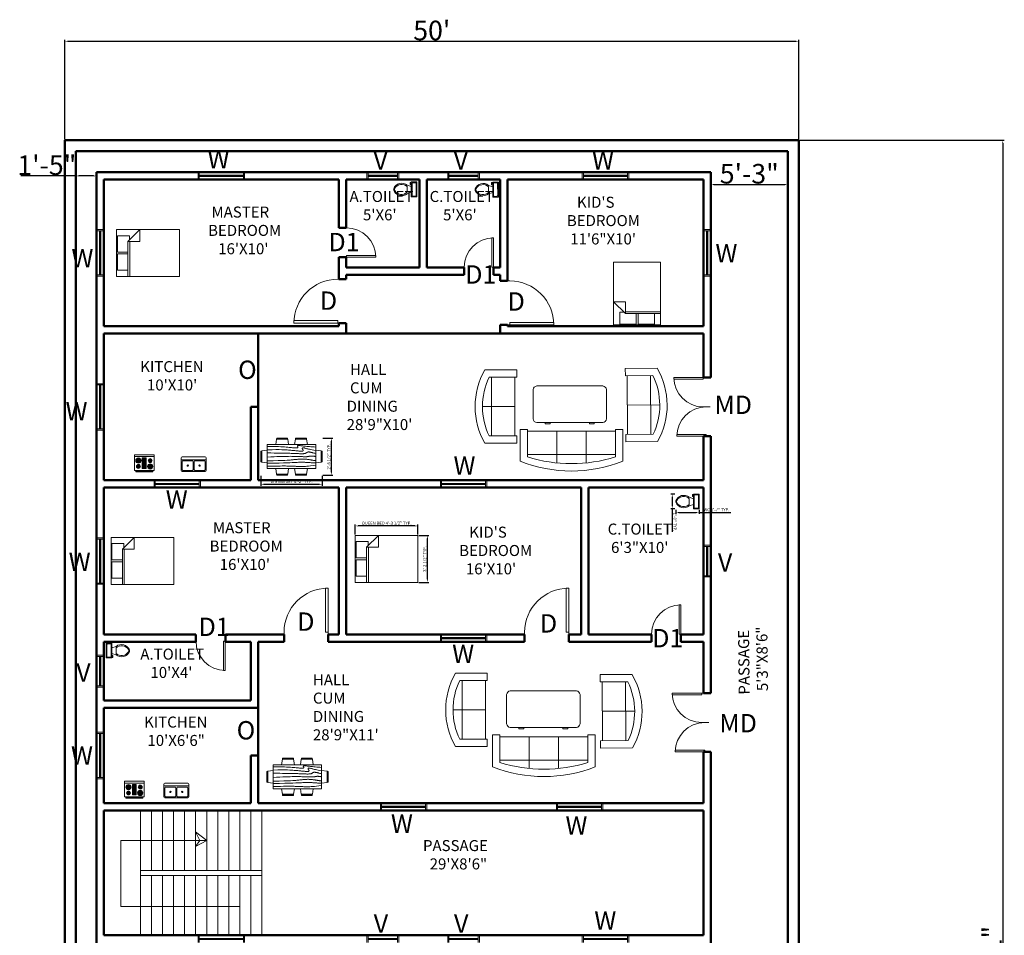
# Model space of a CAD drawing. Units: inches. Extents: x -7040 to -4088, y 6092 to 7645.
# Tile 9 of 11: x -5837 to -5032, y 6864 to 7612. Entities that reach past the tile are written whole.
import ezdxf

# ---------------------------------------------------------------- set-up
doc = ezdxf.new("R2010")
doc.units = ezdxf.units.IN
for name, color, linetype, lineweight in [('A-ANNO-DIMS', 2, 'Continuous', 18), ('A-ANNO-TEXT', 7, 'Continuous', 25), ('A-AREA-IDEN', 3, 'Continuous', 25), ('A-DOOR', 3, 'Continuous', 18), ('A-FLOR-FIXT', 9, 'Continuous', 13), ('A-FLOR-STRS', 2, 'Continuous', 18), ('A-FURN', 8, 'Continuous', 13), ('A-GLAZ', 4, 'Continuous', 18), ('A-WALL', 7, 'Continuous', 50)]:
    doc.layers.add(name, color=color, linetype=linetype, lineweight=lineweight)
doc.styles.get("Standard").update_dxf_attribs({"font": 'arial.ttf'})
doc.dimstyles.new('ISO-25', dxfattribs={"dimtxt": 2.5, "dimasz": 2.5, "dimexe": 1.25, "dimexo": 0.625, "dimtad": 1, "dimdec": 0, "dimlunit": 3, "dimtxsty": 'Standard', "dimcen": 2.5, "dimadec": 0, "dimazin": 0, "dimtfac": 1, "dimtdec": 0, "dimtmove": 0, "dimatfit": 3, "dimfxl": 1, "dimarcsym": 0})

# ---------------------------------------------------------------- blocks, each defined once
blk = doc.blocks.new('*U8')
for p, q in [((0, 0), (0, -100)), ((750, 0), (750, -100))]:
    blk.add_line(p, q)
blk.add_lwpolyline([(0, 0), (0, 750), (43.75, 750), (43.75, 0)], close=True)
blk.add_arc((0, 0), 750, 0, 90)
blk = doc.blocks.new('Bed - Queen')
for p, q in [((0, -80.00003), (0, 0)), ((0, 0), (59.99999, 0)), ((59.99999, 0), (59.99999, -80.00003)), ((7.99999, -1.2), (28.79998, -1.2)), ((7.99999, -14.4), (7.99999, -1.2)), ((28.79998, -1.2), (28.79998, -14.4)), ((31.19999, -1.2), (51.99999, -1.2)), ((31.19999, -14.4), (31.19999, -1.2)), ((51.99999, -1.2), (51.99999, -16.4)), ((0, -14.4), (44.8, -14.4)), ((44.8, -16.8), (0, -16.8)), ((59.99999, -29.6), (44.8, -14.4)), ((44.8, -14.4), (44.8, -29.6)), ((51.99999, -16.4), (46.79936, -16.4)), ((44.8, -29.6), (59.99999, -29.6)), ((59.99999, -80.00003), (0, -80.00003))]:
    blk.add_line(p, q)
blk = doc.blocks.new('Range-Oven - 30 in top')
for p, q in [((0, -3), (30, -3)), ((12, -6), (18, -6)), ((13, -20), (13, -6)), ((14, -6), (14, -20)), ((15, -20), (15, -6)), ((16, -6), (16, -20)), ((17, -20), (17, -6)), ((6, -24), (6, -25)), ((8, -25), (8, -24)), ((18, -20), (12, -20)), ((22, -25), (22, -24)), ((24, -24), (24, -25))]:
    blk.add_line(p, q)
for points in [[(0, -24), (0, 0), (30, 0), (30, -24)], [(12, -21), (12, -5), (18, -5), (18, -21)], [(2, -26), (2, -25), (28, -25), (28, -26)]]:
    blk.add_lwpolyline(points, close=True)
for centre, radius in [((6, -9), 4), ((6, -9), 3), ((6, -18), 3), ((6, -9), 2), ((6, -9), 1), ((24, -18), 4), ((24, -9), 3), ((24, -18), 3), ((24, -9), 2), ((24, -9), 1), ((6, -18), 2), ((6, -18), 1), ((24, -18), 2), ((24, -18), 1)]:
    blk.add_circle(centre, radius)
blk = doc.blocks.new('Sink-double - 36 in top')
for p, q in [((-18, -4), (18, -4)), ((-0.75, -18.5), (-0.75, -6.5)), ((0.75, -6.5), (0.75, -18.5))]:
    blk.add_line(p, q)
for points in [[(-16.5, 0), (16.5, 0)], [(-18, -19.5), (-18, -1.5)], [(-16.5, -18.5), (-16.5, -6.5)], [(-15.5, -5.5), (-1.75, -5.5)], [(1.75, -5.5), (15.5, -5.5)], [(16.5, -6.5), (16.5, -18.5)], [(18, -1.5), (18, -19.5)], [(16.5, -21), (-16.5, -21)], [(-1.75, -19.5), (-15.5, -19.5)], [(15.5, -19.5), (1.75, -19.5)]]:
    blk.add_lwpolyline(points)
for centre, radius in [((-8.5, -12.5), 1), ((-8.5, -12.5), 0.5), ((8.5, -12.5), 1), ((8.5, -12.5), 0.5)]:
    blk.add_circle(centre, radius)
for centre, radius, start, end in [((-16.5, -1.5), 1.5, 90, 180), ((16.5, -1.5), 1.5, 0, 90), ((-15.5, -6.5), 1, 90, 180), ((-1.75, -6.5), 1, 0, 90), ((1.75, -6.5), 1, 90, 180), ((15.5, -6.5), 1, 0, 90), ((-16.5, -19.5), 1.5, 180, 270), ((-15.5, -18.5), 1, 180, 270), ((-1.75, -18.5), 1, 270, 0), ((1.75, -18.5), 1, 180, 270), ((15.5, -18.5), 1, 270, 0), ((16.5, -19.5), 1.5, 270, 0)]:
    blk.add_arc(centre, radius, start, end)
blk = doc.blocks.new('Toilet - top')
for p, q in [((-10, -8.5), (-8, -8.5)), ((-10, -9.5), (-10, -8.5)), ((-7, -9.5), (-10, -9.5)), ((-8, -8.5), (-8, -8)), ((-7, -8), (-7, -9.5)), ((-4, -8), (-6, -14)), ((4, -8), (6, -14)), ((9.5, -6), (9.5, -2)), ((4, -14), (-4, -14))]:
    blk.add_line(p, q)
blk.add_lwpolyline([(10.5, -8), (10.5, 0), (-10.5, 0), (-10.5, -8)], close=True)
for points in [[(-9.5, -2), (-9.5, -6)], [(8.5, -1), (-8.5, -1)], [(-8.5, -7), (8.5, -7)]]:
    blk.add_lwpolyline(points)
for centre, radius, start, end in [((-8.6, -1.9), 0.884, 81.8699, 188.1301), ((-8.6, -6.1), 0.884, 171.8699, 278.1301), ((8.6, -1.9), 0.884, 351.8699, 98.1301), ((8.6, -6.1), 0.884, 261.8699, 8.1301), ((3.5, -21.6), 12.2, 141.4691, 247.9714), ((4.2, -21.8), 11.3, 136.3677, 238.9468), ((-3.5, -21.6), 12.2, 292.0284, 38.5307), ((-4.2, -21.8), 11.3, 301.053, 43.6321), ((0, -27.9), 4, 245.7318, 294.2682), ((0, -29), 4, 254.8605, 285.1395)]:
    blk.add_arc(centre, radius, start, end)
blk = doc.blocks.new('Desk - 30 x 60 in.')
for p, q in [((-26.999995, 0), (26.999995, 0)), ((-29.999995, -27), (-29.999995, -3)), ((29.999995, -3), (29.999995, -27)), ((26.999995, -30), (-26.999995, -30)), ((-20.000005, -30), (-20.000005, -31)), ((-20.000005, -31), (-16.000005, -31)), ((-16.000005, -31), (-16.000005, -30)), ((15.999995, -31), (15.999995, -30)), ((19.999995, -31), (15.999995, -31)), ((19.999995, -30), (19.999995, -31))]:
    blk.add_line(p, q)
for centre, start, end in [((-26.499995, -3.5), 98.1301, 171.8699), ((26.499995, -3.5), 8.130102, 81.8699), ((-26.499995, -26.5), 188.1301, 261.8699), ((26.499995, -26.5), 278.1301, 351.8699)]:
    blk.add_arc(centre, 3.535534, start, end)
blk = doc.blocks.new('Sofa - Roundback 7 ft.')
for p, q in [((-12.00002, -32.4421), (-12.00003, -6.5971)), ((11.99997, -32.4421), (11.99998, -6.5971)), ((-36.000027, -34), (-36.000027, -11.4696)), ((-35.999844, -13.3819), (35.9998, -13.3819)), ((35.99998, -34), (35.99998, -11.4696)), ((-36.000027, -32.4421), (35.99998, -32.4421))]:
    blk.add_line(p, q)
for points in [[(-36.000027, -34), (-42.000027, -34), (-42.000027, -8)], [(41.99998, -8), (41.99998, -34), (35.99998, -34)]]:
    blk.add_lwpolyline(points)
for centre, radius, start, end in [((0, -114.25), 114.25, 68.43141, 111.5686), ((-0.00001, -127.1968), 121.1968, 72.72033, 107.2797)]:
    blk.add_arc(centre, radius, start, end)
blk = doc.blocks.new('Sofa - Roundback Loveseat 5 ft.')
for p, q in [((0, -32.44198), (0, -5.99998)), ((-24, -33.99998), (-24, -11.46958)), ((-23.9998, -13.38178), (23.99986, -13.38178)), ((24.00004, -33.99998), (24.00004, -11.46958)), ((-24, -32.44198), (24.00004, -32.44198))]:
    blk.add_line(p, q)
for points in [[(-24, -33.99998), (-30, -33.99998), (-30, -7.99998)], [(30.00004, -7.99998), (30.00004, -33.99998), (24.00004, -33.99998)]]:
    blk.add_lwpolyline(points)
for centre, radius, start, end in [((0, -60.24998), 60.24998, 60.13715, 119.8628), ((0, -61.38438), 55.38444, 64.32083, 115.6792)]:
    blk.add_arc(centre, radius, start, end)
blk = doc.blocks.new('Dining Set - 36 x 72 in.')
for p, q in [((36, 18), (-36, 18)), ((-36, 18), (-36, -18)), ((-22.2343, 26.00059), (-23.4847, 17.99762)), ((-22.2304, 26), (-5.7608, 26)), ((-22, 27.5), (-22.1562, 26.50042)), ((-5.8416, 26.5), (-22.1534, 26.5)), ((-22, 27.5), (-6, 27.5)), ((-5.8437, 26.49966), (-6, 27.5)), ((-4.5152, 17.99762), (-5.7655, 25.99926)), ((5.7657, 26.00059), (4.5153, 17.99762)), ((5.7696, 26), (22.2392, 26)), ((6, 27.5), (5.8438, 26.50042)), ((22.1584, 26.5), (5.8466, 26.5)), ((6, 27.5), (22, 27.5)), ((22.1563, 26.49966), (22, 27.5)), ((23.4848, 17.99762), (22.2345, 25.99926)), ((36, -18), (36, 18)), ((-45.5, 8), (-44.5004, 8.15617)), ((-45.5, 8), (-45.5, -8)), ((-44.5, -8.15843), (-44.5, 8.15338)), ((-44.0006, 8.23428), (-35.9976, 9.48474)), ((-44, 8.23041), (-44, -8.23915)), ((44.0006, 8.23428), (35.9976, 9.48474)), ((44, 8.23041), (44, -8.23915)), ((44.5, -8.15843), (44.5, 8.15338)), ((45.5, 8), (44.5005, 8.15617)), ((45.5, 8), (45.5, -8)), ((-44.4997, -8.15631), (-45.5, -8)), ((-35.9976, -9.48476), (-43.9993, -8.2345)), ((35.9976, -9.48476), (43.9993, -8.2345)), ((44.4997, -8.15631), (45.5, -8)), ((-36, -18), (36, -18)), ((-22.2343, -26.0006), (-23.4847, -17.99762)), ((-22.2304, -26), (-5.7608, -26)), ((-22, -27.5), (-22.1562, -26.50044)), ((-5.8416, -26.5), (-22.1534, -26.5)), ((-22, -27.5), (-6, -27.5)), ((-5.8437, -26.49967), (-6, -27.5)), ((-4.5152, -17.99762), (-5.7655, -25.99928)), ((5.7657, -26.0006), (4.5153, -17.99762)), ((5.7696, -26), (22.2392, -26)), ((6, -27.5), (5.8438, -26.50044)), ((22.1584, -26.5), (5.8466, -26.5)), ((6, -27.5), (22, -27.5)), ((22.1563, -26.49967), (22, -27.5)), ((23.4848, -17.99762), (22.2345, -25.99928))]:
    blk.add_line(p, q)
for points in [[(-36, 15), (-31.1772, 14.97754), (-26.8079, 14.91406), (-22.8538, 14.81543), (-19.276, 14.6875), (-16.0362, 14.53613), (-13.0957, 14.36718), (-10.4159, 14.18652), (-7.9583, 14), (-5.6904, 13.81315), (-3.6035, 13.63021), (-1.6954, 13.45508), (0.0365, 13.29166), (1.5945, 13.14388), (2.9811, 13.01562), (4.1988, 12.9108), (5.25, 12.83333), (6.1393, 12.78613), (6.8802, 12.76823), (7.4883, 12.77767), (7.9792, 12.8125), (8.3685, 12.87077), (8.6719, 12.95052), (8.9049, 13.0498), (9.0833, 13.16666), (9.2205, 13.29899), (9.3216, 13.44401), (9.3895, 13.59879), (9.4271, 13.76041), (9.4373, 13.92594), (9.4232, 14.09245), (9.3875, 14.257), (9.3333, 14.41666), (9.2638, 14.56917), (9.1836, 14.71484), (9.0975, 14.85465), (9.0104, 14.98958), (8.9272, 15.1206), (8.8529, 15.2487), (8.7922, 15.37483), (8.75, 15.5), (8.7305, 15.62467), (8.7344, 15.74739), (8.7617, 15.86621), (8.8125, 15.97916), (8.8867, 16.08431), (8.9844, 16.17968), (9.1055, 16.26334), (9.25, 16.33333), (9.4189, 16.38802), (9.6172, 16.42708), (9.8506, 16.45052), (10.125, 16.45833), (10.4463, 16.45052), (10.8203, 16.42708), (11.2529, 16.38802), (11.75, 16.33333), (12.3184, 16.26318), (12.9694, 16.17838), (13.7151, 16.07991), (14.5677, 15.96875), (15.5395, 15.84586), (16.6426, 15.71224), (17.8893, 15.56884), (19.2917, 15.41666), (20.859, 15.25667), (22.5879, 15.08984), (24.4721, 14.91715), (26.5052, 14.73958), (28.6809, 14.5581), (30.9929, 14.3737), (33.4347, 14.18733), (36, 14)], [(-36, 10), (-28.9766, 10.14274), (-23.1725, 10.20442), (-18.4241, 10.19775), (-14.5677, 10.13541), (-11.4399, 10.03011), (-8.877, 9.89453), (-6.7154, 9.74137), (-4.7917, 9.58333), (-2.9698, 9.43082), (-1.2246, 9.28515), (0.4415, 9.14534), (2.026, 9.01041), (3.5266, 8.87939), (4.9408, 8.7513), (6.266, 8.62516), (7.5, 8.5), (8.6411, 8.37549), (9.6914, 8.2539), (10.6538, 8.13818), (11.5312, 8.03125), (12.3267, 7.93603), (13.043, 7.85547), (13.6831, 7.79248), (14.25, 7.75), (14.7471, 7.7303), (15.1797, 7.73307), (15.5537, 7.75732), (15.875, 7.80208), (16.1494, 7.86637), (16.3828, 7.94922), (16.5811, 8.04964), (16.75, 8.16666), (16.8944, 8.29915), (17.0143, 8.44531), (17.1089, 8.60319), (17.1771, 8.77083), (17.218, 8.94629), (17.2305, 9.1276), (17.2137, 9.31282), (17.1667, 9.5), (17.0895, 9.6875), (16.987, 9.875), (16.8649, 10.0625), (16.7292, 10.25), (16.5856, 10.4375), (16.4401, 10.625), (16.2985, 10.8125), (16.1667, 11), (16.05, 11.18733), (15.9518, 11.3737), (15.8752, 11.5581), (15.8229, 11.73958), (15.798, 11.91715), (15.8034, 12.08984), (15.842, 12.25667), (15.9167, 12.41666), (16.0295, 12.56836), (16.1784, 12.70833), (16.3605, 12.83268), (16.5729, 12.9375), (16.8127, 13.01888), (17.0768, 13.07291), (17.3625, 13.0957), (17.6667, 13.08333), (17.9894, 13.03312), (18.3418, 12.94726), (18.7382, 12.82918), (19.1927, 12.68229), (19.7195, 12.51001), (20.3327, 12.31575), (21.0465, 12.10294), (21.875, 11.875), (22.8357, 11.63354), (23.959, 11.37304), (25.2786, 11.08618), (26.8282, 10.76562), (28.6414, 10.40405), (30.752, 9.99414), (33.1936, 9.52856), (36, 9)], [(-36, 5.5), (-30.7157, 5.3348), (-26.069, 5.20963), (-21.9946, 5.11767), (-18.4271, 5.05208), (-15.3009, 5.00602), (-12.5508, 4.97265), (-10.1112, 4.94515), (-7.9167, 4.91666), (-5.909, 4.88167), (-4.0586, 4.83984), (-2.3429, 4.79215), (-0.7396, 4.73958), (0.7739, 4.6831), (2.22, 4.6237), (3.6213, 4.56233), (5, 4.5), (6.373, 4.43782), (7.7344, 4.3776), (9.0723, 4.32129), (10.375, 4.27083), (11.6309, 4.22819), (12.8281, 4.19531), (13.9551, 4.17415), (15, 4.16666), (15.954, 4.17448), (16.819, 4.19791), (17.6001, 4.23698), (18.3021, 4.29166), (18.9299, 4.36198), (19.4883, 4.44791), (19.9823, 4.54948), (20.4167, 4.66666), (20.7969, 4.79899), (21.1302, 4.94401), (21.4245, 5.09879), (21.6875, 5.26041), (21.9271, 5.42594), (22.1511, 5.59245), (22.3672, 5.757), (22.5834, 5.91666), (22.8065, 6.06868), (23.0404, 6.21093), (23.2879, 6.34147), (23.5521, 6.45833), (23.8358, 6.55957), (24.142, 6.64323), (24.4735, 6.70735), (24.8334, 6.75), (25.2235, 6.76969), (25.642, 6.76692), (26.0858, 6.74267), (26.5521, 6.69791), (27.0379, 6.63362), (27.5404, 6.55078), (28.0565, 6.45036), (28.5834, 6.33333), (29.1242, 6.19987), (29.7071, 6.04687), (30.3661, 5.87044), (31.1354, 5.66666), (32.0493, 5.43164), (33.142, 5.16146), (34.4475, 4.85221), (36, 4.5)], [(-36, -1), (-30.7915, -0.6591), (-26.0195, -0.38216), (-21.6519, -0.16284), (-17.6563, 0.00521), (-14.0005, 0.12833), (-10.6523, 0.21289), (-7.5796, 0.26522), (-4.75, 0.29166), (-2.134, 0.29793), (0.2878, 0.28711), (2.5317, 0.26163), (4.6146, 0.22396), (6.5529, 0.17651), (8.3633, 0.12174), (10.0623, 0.06209), (11.6667, 0), (13.1899, -0.06201), (14.6341, -0.1211), (15.9982, -0.17432), (17.2813, -0.21875), (18.4823, -0.25147), (19.6003, -0.26953), (20.6343, -0.27002), (21.5834, -0.25), (22.4481, -0.20768), (23.2357, -0.14584), (23.9549, -0.06836), (24.6146, 0.02083), (25.2235, 0.11784), (25.7904, 0.21875), (26.3241, 0.31966), (26.8334, 0.41666), (27.3265, 0.50618), (27.8099, 0.58593), (28.2894, 0.65397), (28.7709, 0.70833), (29.2601, 0.74707), (29.763, 0.76823), (30.2855, 0.76985), (30.8334, 0.75), (31.4088, 0.70784), (31.9994, 0.64713), (32.589, 0.57275), (33.1615, 0.48958), (33.7008, 0.4025), (34.1908, 0.3164), (34.6153, 0.23616), (34.9584, 0.16666), (35.2099, 0.11165), (35.3848, 0.07031), (35.504, 0.04069), (35.5886, 0.02083), (35.6594, 0.00879), (35.7377, 0.0026), (35.8442, 0.00032), (36, 0)], [(-36, -6.5), (-27.1843, -6.31267), (-20.084, -6.1263), (-14.469, -5.9419), (-10.1094, -5.76042), (-6.7752, -5.58285), (-4.2363, -5.41016), (-2.2629, -5.24333), (-0.625, -5.08334), (0.8708, -4.93099), (2.2715, -4.78646), (3.5872, -4.64974), (4.8281, -4.52084), (6.0046, -4.39974), (7.127, -4.28646), (8.2053, -4.18099), (9.25, -4.08334), (10.2705, -3.99382), (11.2734, -3.91407), (12.2647, -3.84603), (13.25, -3.79167), (14.2354, -3.75293), (15.2266, -3.73177), (16.2295, -3.73015), (17.25, -3.75), (18.2912, -3.79248), (19.3451, -3.85547), (20.4009, -3.93604), (21.4479, -4.03125), (22.4754, -4.13819), (23.4727, -4.25391), (24.4289, -4.37549), (25.3334, -4.5), (26.1785, -4.62492), (26.9694, -4.74935), (27.7145, -4.87281), (28.4219, -4.99479), (29.1, -5.11483), (29.7572, -5.23242), (30.4016, -5.34709), (31.0417, -5.45834), (31.6837, -5.56437), (32.3262, -5.65821), (32.9658, -5.73153), (33.599, -5.77604), (34.2224, -5.78345), (34.8327, -5.74545), (35.4264, -5.65373), (36, -5.5)], [(-36, -10), (-26.4022, -9.81299), (-18.4675, -9.62891), (-11.9839, -9.45069), (-6.7396, -9.28125), (-2.5226, -9.12354), (0.8789, -8.98047), (3.6769, -8.85498), (6.0833, -8.75), (8.2767, -8.66765), (10.3021, -8.60677), (12.1712, -8.56543), (13.8958, -8.54167), (15.4876, -8.53353), (16.9583, -8.53907), (18.3197, -8.55632), (19.5834, -8.58334), (20.7616, -8.61841), (21.8685, -8.66081), (22.9188, -8.71004), (23.9271, -8.76563), (24.9081, -8.82707), (25.8763, -8.89388), (26.8465, -8.96558), (27.8334, -9.04167), (28.8474, -9.12118), (29.8828, -9.20117), (30.93, -9.27824), (31.9792, -9.34896), (33.0205, -9.40991), (34.0443, -9.45768), (35.0407, -9.48885), (36, -9.5)], [(-36, -14.5), (-30.0881, -14.33513), (-25.0332, -14.21224), (-20.7312, -14.12647), (-17.0781, -14.07292), (-13.97, -14.04671), (-11.3027, -14.04297), (-8.9724, -14.05681), (-6.875, -14.08334), (-4.9224, -14.11833), (-3.0905, -14.16016), (-1.3709, -14.20785), (0.2448, -14.26042), (1.7647, -14.3169), (3.1973, -14.3763), (4.5507, -14.43767), (5.8333, -14.5), (7.0554, -14.5621), (8.235, -14.62175), (9.3922, -14.67652), (10.5469, -14.72396), (11.7192, -14.76164), (12.929, -14.78711), (14.1965, -14.79794), (15.5417, -14.79167), (16.9933, -14.76424), (18.6152, -14.70508), (20.4804, -14.60197), (22.6615, -14.44271), (25.2312, -14.21509), (28.2624, -13.9069), (31.8277, -13.50594), (36, -13)]]:
    blk.add_lwpolyline(points)
blk = doc.blocks.new('*D99')
at = {"layer": 'A-ANNO-DIMS', "color": 0, "lineweight": -2, "transparency": 16777216}
for p, q in [((-5271.9, 7487.13), (-5271.9, 7476.32)), ((-5208.9, 7487.13), (-5208.9, 7476.32)), ((-5269.4, 7477.57), (-5211.4, 7477.57))]:
    blk.add_line(p, q, dxfattribs=at)
at = {"layer": 'A-ANNO-DIMS', "color": 0, "transparency": 16777216}
for points in [[(-5269.4, 7477.98), (-5269.4, 7477.15), (-5271.9, 7477.57)], [(-5211.4, 7477.98), (-5211.4, 7477.15), (-5208.9, 7477.57)]]:
    blk.add_solid(points, dxfattribs=at)
at = {"layer": 'Defpoints', "color": 0, "transparency": 16777216}
for p in [(-5271.9, 7487.76), (-5208.9, 7487.76), (-5208.9, 7477.57)]:
    blk.add_point(p, dxfattribs=at)
at = {"layer": 'A-ANNO-DIMS', "color": 0, "transparency": 16777216, "insert": (-5240.4, 7486.37), "char_height": 2.5, "attachment_point": 5}
blk.add_mtext('{\\H6.4x;5\'-3"}', dxfattribs=at)
blk = doc.blocks.new('*D100')
at = {"layer": 'A-ANNO-DIMS', "color": 0, "lineweight": -2, "transparency": 16777216}
for p, q in [((-5790.9, 7484.62), (-5835.67, 7484.62)), ((-5790.9, 7487.13), (-5790.9, 7483.37)), ((-5776.4, 7484.62), (-5788.4, 7484.62)), ((-5773.9, 7487.13), (-5773.9, 7483.37))]:
    blk.add_line(p, q, dxfattribs=at)
at = {"layer": 'A-ANNO-DIMS', "color": 0, "transparency": 16777216}
for points in [[(-5788.4, 7485.03), (-5788.4, 7484.2), (-5790.9, 7484.62)], [(-5776.4, 7485.03), (-5776.4, 7484.2), (-5773.9, 7484.62)]]:
    blk.add_solid(points, dxfattribs=at)
at = {"layer": 'Defpoints', "color": 0, "transparency": 16777216}
for p in [(-5790.9, 7487.76), (-5790.9, 7484.62), (-5773.9, 7487.76)]:
    blk.add_point(p, dxfattribs=at)
at = {"layer": 'A-ANNO-DIMS', "color": 0, "transparency": 16777216, "insert": (-5814.54, 7493.41), "char_height": 2.5, "attachment_point": 5}
blk.add_mtext('{\\H6.4x;1\'-5"}', dxfattribs=at)
blk = doc.blocks.new('*D101')
at = {"layer": 'A-ANNO-DIMS', "color": 0, "lineweight": -2, "transparency": 16777216}
for p, q in [((-5799.9, 7514.38), (-5799.9, 7595.96)), ((-5797.4, 7594.71), (-5202.4, 7594.71)), ((-5199.9, 7514.38), (-5199.9, 7595.96))]:
    blk.add_line(p, q, dxfattribs=at)
at = {"layer": 'A-ANNO-DIMS', "color": 0, "transparency": 16777216}
for points in [[(-5797.4, 7595.13), (-5797.4, 7594.29), (-5799.9, 7594.71)], [(-5202.4, 7595.13), (-5202.4, 7594.29), (-5199.9, 7594.71)]]:
    blk.add_solid(points, dxfattribs=at)
at = {"layer": 'Defpoints', "color": 0, "transparency": 16777216}
for p in [(-5199.9, 7594.71), (-5799.9, 7513.76), (-5199.9, 7513.76)]:
    blk.add_point(p, dxfattribs=at)
at = {"layer": 'A-ANNO-DIMS', "color": 0, "transparency": 16777216, "insert": (-5499.9, 7603.5), "char_height": 2.5, "attachment_point": 5}
blk.add_mtext("{\\H6.4x;50'}", dxfattribs=at)
blk = doc.blocks.new('*D102')
at = {"layer": 'A-ANNO-DIMS', "color": 0, "lineweight": -2, "transparency": 16777216}
for p, q in [((-5199.27, 7513.76), (-5031.95, 7513.76)), ((-5033.2, 7511.26), (-5033.2, 6159.26)), ((-5199.27, 6156.76), (-5031.95, 6156.76))]:
    blk.add_line(p, q, dxfattribs=at)
at = {"layer": 'A-ANNO-DIMS', "color": 0, "transparency": 16777216}
for points in [[(-5033.61, 7511.26), (-5032.78, 7511.26), (-5033.2, 7513.76)], [(-5033.61, 6159.26), (-5032.78, 6159.26), (-5033.2, 6156.76)]]:
    blk.add_solid(points, dxfattribs=at)
at = {"layer": 'Defpoints', "color": 0, "transparency": 16777216}
for p in [(-5199.9, 7513.76), (-5199.9, 6156.76), (-5033.2, 6156.76)]:
    blk.add_point(p, dxfattribs=at)
at = {"layer": 'A-ANNO-DIMS', "color": 0, "transparency": 16777216, "insert": (-5042, 6835.26), "char_height": 2.5, "attachment_point": 5, "rotation": 90}
blk.add_mtext('{\\H6.4x;113\'-1"}', dxfattribs=at)
blk = doc.blocks.new('WIN-36')
for p, q in [((0, 6), (0, 0)), ((1, 6), (1, 0)), ((1, 3.5), (37, 3.5)), ((1, 3), (37, 3)), ((1, 2.5), (37, 2.5)), ((37, 6), (37, 0)), ((38, 6), (38, 0))]:
    blk.add_line(p, q)
blk = doc.blocks.new('WIN-24')
for p, q in [((0, 6), (0, 0)), ((1, 6), (1, 0)), ((1, 3.5), (25, 3.5)), ((1, 3), (25, 3)), ((1, 2.5), (25, 2.5)), ((25, 6), (25, 0)), ((26, 6), (26, 0))]:
    blk.add_line(p, q)
blk = doc.blocks.new('*D124')
at = {"layer": 'A-ANNO-DIMS', "color": 0, "lineweight": -2, "transparency": 16777216}
for p, q in [((-5562.45, 7191.37), (-5562.45, 7199.69)), ((-5513.68, 7198.44), (-5559.95, 7198.44)), ((-5511.18, 7191.37), (-5511.18, 7199.69))]:
    blk.add_line(p, q, dxfattribs=at)
at = {"layer": 'A-ANNO-DIMS', "color": 0, "transparency": 16777216}
for points in [[(-5559.95, 7198.86), (-5559.95, 7198.02), (-5562.45, 7198.44)], [(-5513.68, 7198.86), (-5513.68, 7198.02), (-5511.18, 7198.44)]]:
    blk.add_solid(points, dxfattribs=at)
at = {"layer": 'Defpoints', "color": 0, "transparency": 16777216}
for p in [(-5562.45, 7198.44), (-5562.45, 7190.75), (-5511.18, 7190.75)]:
    blk.add_point(p, dxfattribs=at)
at = {"layer": 'A-ANNO-DIMS', "color": 0, "transparency": 16777216, "insert": (-5536.82, 7200.43), "char_height": 2.5, "attachment_point": 5}
blk.add_mtext('QUEEN BED 4\'-3 1/2" TYP.', dxfattribs=at)
blk = doc.blocks.new('*D125')
at = {"layer": 'A-ANNO-DIMS', "color": 0, "lineweight": -2, "transparency": 16777216}
for p, q in [((-5510.56, 7190.75), (-5502.24, 7190.75)), ((-5503.49, 7154.8), (-5503.49, 7188.25)), ((-5510.56, 7152.3), (-5502.24, 7152.3))]:
    blk.add_line(p, q, dxfattribs=at)
at = {"layer": 'A-ANNO-DIMS', "color": 0, "transparency": 16777216}
for points in [[(-5503.91, 7188.25), (-5503.08, 7188.25), (-5503.49, 7190.75)], [(-5503.91, 7154.8), (-5503.08, 7154.8), (-5503.49, 7152.3)]]:
    blk.add_solid(points, dxfattribs=at)
at = {"layer": 'Defpoints', "color": 0, "transparency": 16777216}
for p in [(-5511.18, 7190.75), (-5503.49, 7190.75), (-5511.18, 7152.3)]:
    blk.add_point(p, dxfattribs=at)
at = {"layer": 'A-ANNO-DIMS', "color": 0, "transparency": 16777216, "insert": (-5505.41, 7171.52), "char_height": 2.5, "attachment_point": 5, "rotation": 90}
blk.add_mtext('3\'-2 1/2" TYP.', dxfattribs=at)
blk = doc.blocks.new('*D130')
at = {"layer": 'A-ANNO-DIMS', "color": 0, "lineweight": -2, "transparency": 16777216}
for p, q in [((-5300.49, 7211.69), (-5300.49, 7208.2)), ((-5281.38, 7211.71), (-5281.38, 7208.22)), ((-5297.99, 7209.45), (-5283.88, 7209.47)), ((-5281.38, 7209.47), (-5255.5, 7209.49))]:
    blk.add_line(p, q, dxfattribs=at)
at = {"layer": 'A-ANNO-DIMS', "color": 0, "transparency": 16777216}
for points in [[(-5297.99, 7209.87), (-5297.99, 7209.04), (-5300.49, 7209.45)], [(-5283.88, 7209.88), (-5283.88, 7209.05), (-5281.38, 7209.47)]]:
    blk.add_solid(points, dxfattribs=at)
at = {"layer": 'Defpoints', "color": 0, "transparency": 16777216}
for p in [(-5300.49, 7212.32), (-5281.38, 7212.34), (-5281.38, 7209.47)]:
    blk.add_point(p, dxfattribs=at)
at = {"layer": 'A-ANNO-DIMS', "color": 0, "transparency": 16777216, "insert": (-5267.19, 7211.4), "char_height": 2.5, "attachment_point": 5, "rotation": 0.05144}
blk.add_mtext('WC 1\'-7" TYP.', dxfattribs=at)
blk = doc.blocks.new('*D131')
at = {"layer": 'A-ANNO-DIMS', "color": 0, "lineweight": -2, "transparency": 16777216}
for p, q in [((-5301.12, 7224.46), (-5304.62, 7224.46)), ((-5303.36, 7221.96), (-5303.36, 7214.82)), ((-5301.11, 7212.32), (-5304.6, 7212.31)), ((-5303.35, 7212.32), (-5303.34, 7193.56))]:
    blk.add_line(p, q, dxfattribs=at)
at = {"layer": 'A-ANNO-DIMS', "color": 0, "transparency": 16777216}
for points in [[(-5302.95, 7221.96), (-5303.78, 7221.96), (-5303.37, 7224.46)], [(-5302.94, 7214.82), (-5303.77, 7214.82), (-5303.35, 7212.32)]]:
    blk.add_solid(points, dxfattribs=at)
at = {"layer": 'Defpoints', "color": 0, "transparency": 16777216}
for p in [(-5300.5, 7224.46), (-5303.35, 7212.32), (-5300.49, 7212.32)]:
    blk.add_point(p, dxfattribs=at)
at = {"layer": 'A-ANNO-DIMS', "color": 0, "transparency": 16777216, "insert": (-5301.44, 7201.69), "char_height": 2.5, "attachment_point": 5, "rotation": 270.05144}
blk.add_mtext('1\'-0" TYP.', dxfattribs=at)
blk = doc.blocks.new('*D144')
at = {"layer": 'A-ANNO-DIMS', "color": 0, "lineweight": -2, "transparency": 16777216}
for p, q in [((-5639.56, 7239.42), (-5639.56, 7231.28)), ((-5589.45, 7239.42), (-5589.45, 7231.28)), ((-5637.06, 7232.53), (-5591.95, 7232.53))]:
    blk.add_line(p, q, dxfattribs=at)
at = {"layer": 'A-ANNO-DIMS', "color": 0, "transparency": 16777216}
for points in [[(-5637.06, 7232.94), (-5637.06, 7232.11), (-5639.56, 7232.53)], [(-5591.95, 7232.94), (-5591.95, 7232.11), (-5589.45, 7232.53)]]:
    blk.add_solid(points, dxfattribs=at)
at = {"layer": 'Defpoints', "color": 0, "transparency": 16777216}
for p in [(-5639.56, 7240.04), (-5589.45, 7240.04), (-5589.45, 7232.53)]:
    blk.add_point(p, dxfattribs=at)
at = {"layer": 'A-ANNO-DIMS', "color": 0, "transparency": 16777216, "insert": (-5614.5, 7234.44), "char_height": 2.5, "attachment_point": 5}
blk.add_mtext('DINING SET 4\'-2" TYP.', dxfattribs=at)
blk = doc.blocks.new('*D145')
at = {"layer": 'A-ANNO-DIMS', "color": 0, "lineweight": -2, "transparency": 16777216}
for p, q in [((-5588.82, 7270.33), (-5580.68, 7270.33)), ((-5581.93, 7242.54), (-5581.93, 7267.83)), ((-5588.82, 7240.04), (-5580.68, 7240.04))]:
    blk.add_line(p, q, dxfattribs=at)
at = {"layer": 'A-ANNO-DIMS', "color": 0, "transparency": 16777216}
for points in [[(-5582.35, 7267.83), (-5581.51, 7267.83), (-5581.93, 7270.33)], [(-5582.35, 7242.54), (-5581.51, 7242.54), (-5581.93, 7240.04)]]:
    blk.add_solid(points, dxfattribs=at)
at = {"layer": 'Defpoints', "color": 0, "transparency": 16777216}
for p in [(-5589.45, 7270.33), (-5581.93, 7270.33), (-5589.45, 7240.04)]:
    blk.add_point(p, dxfattribs=at)
at = {"layer": 'A-ANNO-DIMS', "color": 0, "transparency": 16777216, "insert": (-5583.85, 7255.19), "char_height": 2.5, "attachment_point": 5, "rotation": 90}
blk.add_mtext('2\'-6 1/2" TYP.', dxfattribs=at)

msp = doc.modelspace()

# ---------------------------------------------------------------- linework, layer by layer
at = {"layer": 'A-FLOR-STRS'}
for p, q in [((-5737.9, 6863.76), (-5737.9, 6965.76)), ((-5728.9, 6916.76), (-5728.9, 6965.76)), ((-5719.9, 6916.76), (-5719.9, 6965.76)), ((-5710.9, 6916.76), (-5710.9, 6965.76)), ((-5701.9, 6916.76), (-5701.9, 6965.76)), ((-5692.9, 6916.76), (-5692.9, 6965.76)), ((-5683.9, 6916.76), (-5683.9, 6965.76)), ((-5674.9, 6916.76), (-5674.9, 6965.76)), ((-5665.9, 6916.76), (-5665.9, 6965.76)), ((-5656.9, 6916.76), (-5656.9, 6965.76)), ((-5647.9, 6916.76), (-5647.9, 6965.76)), ((-5638.9, 6863.76), (-5638.9, 6965.76)), ((-5683.9, 6941.26), (-5692.9, 6948.41)), ((-5692.9, 6948.41), (-5689.59, 6941.26)), ((-5683.9, 6941.26), (-5754.05, 6941.26)), ((-5754.05, 6941.26), (-5754.05, 6887.3)), ((-5689.59, 6941.26), (-5692.9, 6936.41)), ((-5692.9, 6936.41), (-5683.9, 6941.26)), ((-5737.9, 6916.76), (-5638.9, 6916.76)), ((-5737.9, 6912.76), (-5638.9, 6912.76)), ((-5728.9, 6863.76), (-5728.9, 6912.76)), ((-5719.9, 6863.76), (-5719.9, 6912.76)), ((-5710.9, 6863.76), (-5710.9, 6912.76)), ((-5701.9, 6863.76), (-5701.9, 6912.76)), ((-5692.9, 6863.76), (-5692.9, 6912.76)), ((-5683.9, 6863.76), (-5683.9, 6912.76)), ((-5674.9, 6863.76), (-5674.9, 6912.76)), ((-5665.9, 6863.76), (-5665.9, 6912.76)), ((-5656.9, 6863.76), (-5656.9, 6912.76)), ((-5647.9, 6863.76), (-5647.9, 6912.76)), ((-5754.05, 6887.3), (-5656.9, 6887.3))]:
    msp.add_line(p, q, dxfattribs=at)
at = {"layer": 'A-WALL'}
for p, q in [((-5799.9, 7513.76), (-5199.9, 7513.76)), ((-5799.9, 6156.76), (-5799.9, 7513.76)), ((-5199.9, 7513.76), (-5199.9, 6156.76)), ((-5790.9, 6165.76), (-5790.9, 7504.76)), ((-5790.9, 7504.76), (-5208.9, 7504.76)), ((-5208.9, 7504.76), (-5208.9, 6165.76)), ((-5773.9, 6182.76), (-5773.9, 7487.76)), ((-5773.9, 7487.76), (-5271.9, 7487.76)), ((-5271.9, 7487.76), (-5271.9, 7319.76)), ((-5767.9, 7481.76), (-5575.9, 7481.76)), ((-5767.9, 7361.76), (-5767.9, 7481.76)), ((-5575.9, 7442.17), (-5575.9, 7481.76)), ((-5575.9, 7442.17), (-5575.9, 7481.76)), ((-5569.9, 7481.76), (-5509.9, 7481.76)), ((-5569.9, 7442.17), (-5569.9, 7481.76)), ((-5569.9, 7442.17), (-5569.9, 7481.76)), ((-5509.9, 7409.76), (-5509.9, 7481.76)), ((-5503.9, 7409.76), (-5503.9, 7481.76)), ((-5503.9, 7481.76), (-5443.9, 7481.76)), ((-5443.9, 7409.76), (-5443.9, 7481.76)), ((-5437.9, 7481.76), (-5277.9, 7481.76)), ((-5437.9, 7398.73), (-5437.9, 7481.76)), ((-5277.9, 7481.76), (-5277.9, 7361.76)), ((-5575.9, 7442.17), (-5569.9, 7442.17)), ((-5575.9, 7418.17), (-5569.9, 7418.17)), ((-5575.9, 7400.19), (-5575.9, 7418.17)), ((-5575.9, 7400.19), (-5575.9, 7418.17)), ((-5569.9, 7409.76), (-5569.9, 7418.17)), ((-5569.9, 7409.76), (-5569.9, 7418.17)), ((-5569.9, 7409.76), (-5509.9, 7409.76)), ((-5503.9, 7409.76), (-5473.4, 7409.76)), ((-5473.4, 7409.76), (-5473.4, 7403.76)), ((-5449.4, 7409.76), (-5449.4, 7403.76)), ((-5449.4, 7409.76), (-5443.9, 7409.76)), ((-5575.9, 7400.19), (-5569.9, 7400.19)), ((-5569.9, 7403.76), (-5509.9, 7403.76)), ((-5569.9, 7400.19), (-5569.9, 7403.76)), ((-5569.9, 7400.19), (-5569.9, 7403.76)), ((-5509.9, 7403.76), (-5473.4, 7403.76)), ((-5449.4, 7403.76), (-5443.9, 7403.76)), ((-5443.9, 7398.73), (-5443.9, 7403.76)), ((-5443.9, 7398.73), (-5437.9, 7398.73)), ((-5575.9, 7361.76), (-5575.9, 7364.19)), ((-5575.9, 7361.76), (-5575.9, 7364.19)), ((-5575.9, 7364.19), (-5569.9, 7364.19)), ((-5569.9, 7355.76), (-5569.9, 7364.19)), ((-5569.9, 7355.76), (-5569.9, 7364.19)), ((-5767.9, 7361.76), (-5575.9, 7361.76)), ((-5767.9, 7355.76), (-5641.9, 7355.76)), ((-5767.9, 7235.76), (-5767.9, 7355.76)), ((-5641.9, 7355.76), (-5277.9, 7355.76)), ((-5641.9, 7295.76), (-5641.9, 7355.76)), ((-5443.9, 7355.76), (-5443.9, 7362.73)), ((-5443.9, 7362.73), (-5437.9, 7362.73)), ((-5437.9, 7361.76), (-5437.9, 7362.73)), ((-5437.9, 7361.76), (-5277.9, 7361.76)), ((-5277.9, 7355.76), (-5277.9, 7319.76)), ((-5277.9, 7319.76), (-5271.9, 7319.76)), ((-5647.9, 7235.76), (-5647.9, 7295.76)), ((-5647.9, 7235.76), (-5647.9, 7295.76)), ((-5641.9, 7295.76), (-5647.9, 7295.76)), ((-5641.9, 7235.76), (-5641.9, 7295.76)), ((-5641.9, 7235.76), (-5641.9, 7295.76)), ((-5277.9, 7271.76), (-5271.9, 7271.76)), ((-5277.9, 7271.76), (-5277.9, 7235.76)), ((-5271.9, 7271.76), (-5271.9, 7061.76)), ((-5767.9, 7235.76), (-5647.9, 7235.76)), ((-5641.9, 7235.76), (-5277.9, 7235.76)), ((-5767.9, 7229.76), (-5575.9, 7229.76)), ((-5767.9, 7109.76), (-5767.9, 7229.76)), ((-5575.9, 7109.76), (-5575.9, 7229.76)), ((-5569.9, 7109.76), (-5569.9, 7229.76)), ((-5569.9, 7229.76), (-5377.9, 7229.76)), ((-5377.9, 7109.76), (-5377.9, 7229.76)), ((-5371.9, 7109.76), (-5371.9, 7229.76)), ((-5371.9, 7229.76), (-5277.9, 7229.76)), ((-5277.9, 7229.76), (-5277.9, 7109.76)), ((-5767.9, 7109.76), (-5692.63, 7109.76)), ((-5692.63, 7109.76), (-5692.63, 7103.76)), ((-5668.63, 7109.76), (-5668.63, 7103.76)), ((-5668.63, 7109.76), (-5620.66, 7109.76)), ((-5620.66, 7109.76), (-5620.66, 7103.76)), ((-5584.66, 7109.76), (-5584.66, 7103.76)), ((-5584.66, 7109.76), (-5575.9, 7109.76)), ((-5569.9, 7109.76), (-5424, 7109.76)), ((-5424, 7109.76), (-5424, 7103.76)), ((-5388, 7109.76), (-5388, 7103.76)), ((-5388, 7109.76), (-5377.9, 7109.76)), ((-5371.9, 7109.76), (-5320.32, 7109.76)), ((-5320.32, 7109.76), (-5320.32, 7103.76)), ((-5296.32, 7109.76), (-5296.32, 7103.76)), ((-5296.32, 7109.76), (-5277.9, 7109.76)), ((-5767.9, 7103.76), (-5692.63, 7103.76)), ((-5767.9, 7055.76), (-5767.9, 7103.76)), ((-5668.63, 7103.76), (-5647.9, 7103.76)), ((-5647.9, 7055.76), (-5647.9, 7103.76)), ((-5641.9, 7103.76), (-5620.66, 7103.76)), ((-5641.9, 7049.76), (-5641.9, 7103.76)), ((-5584.66, 7103.76), (-5424, 7103.76)), ((-5388, 7103.76), (-5320.32, 7103.76)), ((-5296.32, 7103.76), (-5277.9, 7103.76)), ((-5277.9, 7103.76), (-5277.9, 7061.76)), ((-5277.9, 7061.76), (-5271.9, 7061.76)), ((-5767.9, 7055.76), (-5647.9, 7055.76)), ((-5767.9, 7049.76), (-5641.9, 7049.76)), ((-5767.9, 6971.76), (-5767.9, 7049.76)), ((-5641.9, 7010.76), (-5641.9, 7049.76)), ((-5647.9, 6971.76), (-5647.9, 7010.76)), ((-5647.9, 7010.76), (-5641.9, 7010.76)), ((-5641.9, 6971.76), (-5641.9, 7010.76)), ((-5277.9, 7013.76), (-5271.9, 7013.76)), ((-5277.9, 7013.76), (-5277.9, 6971.76)), ((-5271.9, 7013.76), (-5271.9, 6557.18)), ((-5767.9, 6971.76), (-5647.9, 6971.76)), ((-5641.9, 6971.76), (-5277.9, 6971.76)), ((-5767.9, 6965.76), (-5277.9, 6965.76)), ((-5767.9, 6863.76), (-5767.9, 6965.76)), ((-5277.9, 6965.76), (-5277.9, 6863.76)), ((-5767.9, 6863.76), (-5277.9, 6863.76))]:
    msp.add_line(p, q, dxfattribs=at)

# ---------------------------------------------------------------- block references
at = {"layer": 'A-DOOR'}
for p, xscale, yscale, zscale, rotation in [((-5569.7, 7418.17), -0.0320000014720848, 0.0320000014720848, 0.0320000014720848, 270), ((-5576.58, 7364.19), 0.0479999999999998, 0.0479999999999998, 0.0479999999999998, 90), ((-5436.1, 7362.73), -0.0480000008832502, 0.0480000008832502, 0.0480000008832502, 270), ((-5278.02, 7319.8), -0.032106775189528, 0.032106775189528, 0.032106775189528, 90), ((-5275.55, 7271.73), 0.0321136266787739, 0.0321136266787739, 0.0321136266787739, 90.00000000000003), ((-5668.65, 7104.27), 0.0319325753922831, 0.0319325753922831, 0.0319325753922831, 180), ((-5279.24, 7061.77), -0.032106775189528, 0.032106775189528, 0.032106775189528, 90), ((-5276.77, 7013.69), 0.0321136266787739, 0.0321136266787739, 0.0321136266787739, 90.00000000000003)]:
    msp.add_blockref('*U8', p, dxfattribs=dict(at, xscale=xscale, yscale=yscale, zscale=zscale, rotation=rotation))
for p, xscale, yscale, zscale in [((-5449.4, 7409.96), -0.0319999999999999, 0.0319999999999999, 0.0319999999999999), ((-5584.66, 7111.56), -0.047999997308417, 0.047999997308417, 0.047999997308417), ((-5388, 7111.56), -0.047999997308417, 0.047999997308417, 0.047999997308417), ((-5296.32, 7109.96), -0.0320000011083999, 0.0320000011083999, 0.0320000011083999)]:
    msp.add_blockref('*U8', p, dxfattribs=dict(at, xscale=xscale, yscale=yscale, zscale=zscale))
at = {"layer": 'A-FLOR-FIXT', "xscale": 0.5781895628236116, "yscale": 0.5781895628236116, "zscale": 0.5781895628236116}
for p, rotation in [((-5512.01, 7473.57), 270.0514378338742), ((-5445.47, 7473.41), 270.0514378338742), ((-5281.39, 7218.41), 270.0514378338742), ((-5766.03, 7096.6), 89.40198668992271)]:
    msp.add_blockref('Toilet - top', p, dxfattribs=dict(at, rotation=rotation))
at = {"layer": 'A-FLOR-FIXT'}
for name, p, xscale, yscale, zscale in [('Range-Oven - 30 in top', (-5742.91, 7256.7), 0.5343739847293781, 0.5343739847293781, 0.5343739847293781), ('Sink-double - 36 in top', (-5694.51, 7254.87), 0.5691595575351838, 0.5691595575351838, 0.5691595575351838), ('Range-Oven - 30 in top', (-5751.01, 6989.74), 0.5343739847293781, 0.5343739847293781, 0.5343739847293781), ('Sink-double - 36 in top', (-5708.69, 6988.14), 0.5691595575351838, 0.5691595575351838, 0.5691595575351838)]:
    msp.add_blockref(name, p, dxfattribs=dict(at, xscale=xscale, yscale=yscale, zscale=zscale))
at = {"layer": 'A-FURN', "xscale": 0.6408536689007259, "yscale": 0.6408536689007259, "zscale": 0.6408536689007259}
for p, rotation in [((-5757.5, 7402.41), 90), ((-5312.86, 7362.77), 180), ((-5762.05, 7150.66), 90), ((-5562.45, 7152.3), 90)]:
    msp.add_blockref('Bed - Queen', p, dxfattribs=dict(at, rotation=rotation))
at = {"layer": 'A-FURN'}
for name, p, rotation in [('Sofa - Roundback Loveseat 5 ft.', (-5464.47, 7296), 90.00814269742376), ('Sofa - Roundback Loveseat 5 ft.', (-5307.54, 7297.48), 270.3571450594314), ('Sofa - Roundback 7 ft.', (-5385.75, 7243.36), 179.9884368603272), ('Sofa - Roundback Loveseat 5 ft.', (-5488.53, 7048.07), 90.00814269742376), ('Sofa - Roundback Loveseat 5 ft.', (-5328.06, 7047.1), 270.3571450594314), ('Sofa - Roundback 7 ft.', (-5408.24, 6993.55), 179.9884368603272)]:
    msp.add_blockref(name, p, dxfattribs=dict(at, rotation=rotation))
for p in [(-5387.1, 7312.91), (-5408.7, 7063.64)]:
    msp.add_blockref('Desk - 30 x 60 in.', p, dxfattribs=at)
at = {"layer": 'A-FURN', "xscale": 0.5507153893551977, "yscale": 0.5507153893551977, "zscale": 0.5507153893551977}
for p in [(-5614.5, 7255.19), (-5609.74, 6993.34)]:
    msp.add_blockref('Dining Set - 36 x 72 in.', p, dxfattribs=at)
at = {"layer": 'A-GLAZ'}
for p in [(-5690.9, 7481.76), (-5376.9, 7481.76), (-5726.9, 7229.76), (-5492.9, 7229.76), (-5492.9, 7103.76), (-5541.9, 6965.76), (-5398.07, 6965.76), (-5690.9, 6857.76), (-5376.9, 6857.76)]:
    msp.add_blockref('WIN-36', p, dxfattribs=at)
for name, p, rotation in [('WIN-24', (-5526.9, 7487.76), 180), ('WIN-24', (-5460.9, 7487.76), 180), ('WIN-36', (-5767.9, 7402.76), 89.99999999999775), ('WIN-36', (-5271.9, 7402.76), 90.00000000000082), ('WIN-36', (-5767.9, 7276.76), 89.99999999999775), ('WIN-36', (-5767.9, 7150.76), 90.00000000000126), ('WIN-24', (-5277.9, 7182.76), 269.9999999999933), ('WIN-24', (-5773.9, 7092.76), 269.9999999999962), ('WIN-36', (-5767.9, 6991.76), 89.99999999999817), ('WIN-24', (-5526.9, 6863.76), 180), ('WIN-24', (-5460.9, 6863.76), 180)]:
    msp.add_blockref(name, p, dxfattribs=dict(at, rotation=rotation))

# ---------------------------------------------------------------- texts
at = {"layer": 'A-ANNO-TEXT', "char_height": 15, "attachment_point": 1}
for s, insert in [('{W}', (-5683.2, 7505.71)), ('{V}', (-5547.66, 7504.8)), ('{V}', (-5482.06, 7504.8)), ('{W}', (-5368.95, 7504.84)), ('{D1}', (-5584.34, 7438.05)), ('{W}', (-5268.06, 7428.91)), ('{W}', (-5794.42, 7424.78)), ('{D1}', (-5472.54, 7411.53)), ('{D}', (-5591.32, 7390.14)), ('{D}', (-5437.92, 7389.46)), ('{O}', (-5658.19, 7333.62)), ('{W}', (-5799.25, 7299.87)), ('{MD}', (-5268.87, 7304.97)), ('{W}', (-5482.16, 7255.34)), ('{W}', (-5717.36, 7227.48)), ('{W}', (-5796.7, 7176.61)), ('{V}', (-5266.06, 7176.14)), ('{D1}', (-5690.48, 7123.46)), ('{D}', (-5609.85, 7127.71)), ('{D}', (-5411.51, 7126.27)), ('{D1}', (-5319.74, 7114.18)), ('{W}', (-5483.24, 7101.35)), ('{V}', (-5790.53, 7086.24)), ('{MD}', (-5264.86, 7044.68)), ('{O}', (-5659.39, 7038.9)), ('{W}', (-5794.81, 7018.17)), ('{W}', (-5533.31, 6962.53)), ('{W}', (-5390.65, 6961.14)), ('{W}', (-5367.05, 6883.34)), ('{V}', (-5547.35, 6880.8)), ('{V}', (-5481.74, 6880.8))]:
    msp.add_mtext_dynamic_manual_height_columns(s, width=1030.7133, gutter_width=12.5, heights=[0], dxfattribs=dict(at, insert=insert))
at = {"layer": 'A-AREA-IDEN', "char_height": 9, "attachment_point": 1}
for s, insert in [("{ A.TOILET\\P     5'X6'}", (-5569.89, 7472.29)), ("{C.TOILET\\P    5'X6'}", (-5501.68, 7472.29)), ('{     KID\'S\\P  BEDROOM\\P   11\'6"X10\'}', (-5395, 7467.58)), ("{ MASTER\\PBEDROOM\\P   16'X10'}", (-5682.73, 7459.57)), ("{KITCHEN\\P  10'X10'}", (-5738.19, 7333.2)), ('{  HALL\\P  CUM\\P DINING\\P 28\'9"X10\'}', (-5572.25, 7330.84)), ("{ MASTER\\PBEDROOM\\P   16'X10'}", (-5681.49, 7201.48)), ("{   KID'S\\PBEDROOM\\P  16'X10'}", (-5477.54, 7197.86)), ('{C.TOILET\\P 6\'3"X10\'}', (-5356.14, 7200.37)), ("{A.TOILET\\P   10'X4'}", (-5738.12, 7098.15)), ('{ HALL\\P CUM\\P DINING\\P 28\'9"X11\'}', (-5599.81, 7077.19)), ('{ KITCHEN\\P  10\'X6\'6"}', (-5737.82, 7042.58)), ('{ PASSAGE\\P   29\'X8\'6"}', (-5509.86, 6941.62))]:
    msp.add_mtext_dynamic_manual_height_columns(s, width=1231.1944, gutter_width=12.5, heights=[0], dxfattribs=dict(at, insert=insert))
at = {"layer": 'A-AREA-IDEN', "insert": (-5249.04, 7060.44), "char_height": 9, "attachment_point": 1, "rotation": 90.62104}
msp.add_mtext_dynamic_manual_height_columns('{PASSAGE\\P 5\'3"X8\'6"}', width=1231.1944, gutter_width=12.5, heights=[0], dxfattribs=at)

# ---------------------------------------------------------------- dimensions: what is measured, and where the dimension line sits
at = {"layer": 'A-ANNO-DIMS'}
for base, p1, p2, text, override, picture, middle in [((-5199.9, 7594.71), (-5799.9, 7513.76), (-5199.9, 7513.76), '{\\H6.4x;<>}', {"dimclrd": 0, "dimclre": 0, "dimclrt": 0}, '*D101', (-5499.9, 7603.5)), ((-5790.9, 7484.62), (-5773.9, 7487.76), (-5790.9, 7487.76), '{\\H6.4x;<>}', {"dimclrd": 0, "dimclre": 0, "dimclrt": 0}, '*D100', (-5814.54, 7493.41)), ((-5208.9, 7477.57), (-5271.9, 7487.76), (-5208.9, 7487.76), '{\\H6.4x;<>}', {"dimclrd": 0, "dimclre": 0, "dimclrt": 0}, '*D99', (-5240.4, 7486.37)), ((-5589.45, 7232.53), (-5639.56, 7240.04), (-5589.45, 7240.04), 'DINING SET <> TYP.', {"dimdec": 1, "dimrnd": 0, "dimzin": 1, "dimlunit": 4, "dimfrac": 2}, '*D144', (-5614.5, 7234.44))]:
    dim = msp.add_linear_dim(base=base, p1=p1, p2=p2, text=text, dimstyle='ISO-25', override=override, dxfattribs=at)
    dim.commit()
    dim.dimension.update_dxf_attribs({"geometry": picture, "text_midpoint": middle})
for base, p1, p2, angle, text, override, picture, middle in [((-5033.2, 6156.76), (-5199.9, 7513.76), (-5199.9, 6156.76), 90, '{\\H6.4x;<>}', {"dimclrd": 0, "dimclre": 0, "dimclrt": 0}, '*D102', (-5042, 6835.26)), ((-5581.93, 7270.33), (-5589.45, 7240.04), (-5589.45, 7270.33), 90, '<> TYP.', {"dimdec": 1, "dimrnd": 0, "dimzin": 1, "dimlunit": 4, "dimfrac": 2}, '*D145', (-5583.85, 7255.19)), ((-5303.35, 7212.32), (-5300.5, 7224.46), (-5300.49, 7212.32), 270.05144, '<> TYP.', {"dimdec": 1, "dimrnd": 0, "dimzin": 1, "dimlunit": 4, "dimfrac": 2}, '*D131', (-5301.44, 7201.69)), ((-5281.38, 7209.47), (-5300.49, 7212.32), (-5281.38, 7212.34), 0.05144, 'WC <> TYP.', {"dimdec": 1, "dimrnd": 0, "dimzin": 1, "dimlunit": 4, "dimfrac": 2}, '*D130', (-5267.19, 7211.4)), ((-5562.45, 7198.44), (-5511.18, 7190.75), (-5562.45, 7190.75), 180, 'QUEEN BED <> TYP.', {"dimdec": 1, "dimrnd": 0, "dimzin": 1, "dimlunit": 4, "dimfrac": 2}, '*D124', (-5536.82, 7200.43)), ((-5503.4935, 7190.7499), (-5511.1838, 7152.2987), (-5511.1838, 7190.7499), 90, '<> TYP.', {"dimdec": 1, "dimrnd": 0, "dimzin": 1, "dimlunit": 4, "dimfrac": 2}, '*D125', (-5505.412, 7171.5243))]:
    dim = msp.add_linear_dim(base=base, p1=p1, p2=p2, angle=angle, text=text, dimstyle='ISO-25', override=override, dxfattribs=at)
    dim.commit()
    dim.dimension.update_dxf_attribs({"geometry": picture, "text_midpoint": middle})

doc.saveas('drawing.dxf')
